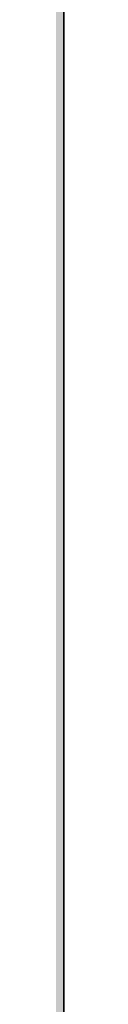
# Model space of a CAD drawing. Units: inches. Extents: x 2091 to 2899, y 967 to 2217.
# Tile 75 of 256: x 2212 to 2212, y 1105 to 1114. Entities that reach past the tile are written whole.
import ezdxf

# ---------------------------------------------------------------- set-up
doc = ezdxf.new("R2010")
doc.units = ezdxf.units.IN
doc.layers.add('A-WALL', color=7, linetype='Continuous', lineweight=35)
doc.layers.add('A-WALL-PATT', color=141, linetype='Continuous', lineweight=13, true_color=0xadddf7)

msp = doc.modelspace()

# ---------------------------------------------------------------- hatches: boundary and pattern name
at = {"layer": 'A-WALL-PATT'}
h = msp.add_hatch(color=256, dxfattribs=at)
h.dxf.hatch_style = 1
h.paths.add_polyline_path([(2212.1436, 1941.4191), (2387.6436, 1941.4191), (2387.6436, 1824.4191), (2392.1436, 1824.4191), (2392.1436, 1941.4191), (2609.6436, 1941.4191), (2609.6436, 1825.9191), (2614.1436, 1825.9191), (2614.1436, 1941.4191), (2794.1436, 1941.4191), (2794.1436, 1928.7622), (2803.1436, 1928.7622), (2803.1436, 2050.9191), (2203.1436, 2050.9191), (2203.1436, 1900.7579), (2212.1436, 1900.7579)])
h.paths.add_polyline_path([(2212.1436, 1945.9191), (2212.1436, 2041.9191), (2794.1436, 2041.9191), (2794.1436, 1945.9191), (2402.2482, 1945.9191), (2401.1024, 1945.7758), (2398.7024, 1945.7758)], flags=16)
h.paths.add_polyline_path([(2230.2299, 1948.0628), (2227.3499, 1949.5028), (2225.9099, 1951.9028), (2223.9899, 1952.8628), (2223.0299, 1955.2628), (2222.0699, 1959.5828), (2222.0699, 1963.4228), (2223.0299, 1965.6628), (2223.9899, 1965.3428), (2225.5859, 1963.8607), (2226.9115, 1964.9573), (2226.9489, 1965.9388), (2227.7783, 1966.9521), (2228.1999, 1968.8787), (2230.7099, 1964.8628), (2233.5899, 1966.3028), (2233.6073, 1966.3319), (2233.7727, 1964.9382), (2234.6338, 1963.6765), (2235.0299, 1963.9028), (2236.282, 1965.5724), (2235.9899, 1962.9428), (2237.9545, 1957.54), (2238.3899, 1957.9028), (2239.2159, 1960.3058), (2238.6546, 1966.385), (2238.6928, 1966.4381), (2238.8406, 1967.4997), (2238.7803, 1967.6875), (2238.8805, 1967.7868), (2238.6669, 1966.2518), (2239.2159, 1960.3058), (2238.3899, 1957.9028), (2236.9499, 1956.7028), (2234.5499, 1949.9828)], flags=0)
h.paths.add_polyline_path([(2278.012, 1948.0628), (2276.4964, 1947.8733), (2275.8498, 1947.6886), (2274.652, 1947.1028)], flags=0)
h.paths.add_polyline_path([(2269.852, 1955.7428), (2268.2762, 1956.6293), (2270.8673, 1956.3484), (2269.372, 1958.1428), (2268.715, 1959.1923), (2270.5698, 1958.7286), (2268.5807, 1961.9061), (2270.812, 1960.8919), (2270.812, 1963.4228), (2271.3933, 1964.7793), (2270.2918, 1966.1562), (2271.772, 1965.6628), (2272.1414, 1966.5248), (2273.9298, 1965.9286), (2275.6304, 1968.0543), (2276.3319, 1966.7219), (2276.5204, 1966.9521), (2276.942, 1968.8787), (2277.7343, 1967.6111), (2278.1399, 1969.4645), (2279.6591, 1967.0337), (2280.412, 1966.7828), (2280.9493, 1967.5888), (2281.6098, 1967.3686), (2282.1333, 1968.1538), (2282.3492, 1966.3334), (2282.3498, 1966.3326), (2283.4076, 1968.0954), (2283.7126, 1965.524), (2284.3202, 1964.6338), (2284.5118, 1964.8892), (2284.235, 1965.7048), (2284.5005, 1967.319), (2284.9079, 1965.4174), (2285.3963, 1966.0686), (2285.4328, 1966.2906), (2285.4733, 1966.1713), (2286.3539, 1967.3454), (2286.222, 1966.1582), (2287.6635, 1968.0802), (2287.714, 1968.4428), (2288.4816, 1969.0167), (2288.574, 1968.7289), (2288.9175, 1969.069), (2288.6068, 1966.8376), (2288.9287, 1963.3513), (2288.935, 1963.3568), (2288.9297, 1963.3404), (2289.0153, 1962.4139), (2290.1112, 1963.8751), (2290.1328, 1963.9426), (2290.2177, 1964.0171), (2290.1112, 1963.8751), (2289.1558, 1960.8916), (2288.594, 1959.2572), (2288.572, 1959.1028), (2289.532, 1960.5428), (2290.012, 1962.4628), (2290.1918, 1962.6427), (2289.7698, 1959.6886), (2286.8898, 1957.2886), (2284.4898, 1950.5686), (2283.3147, 1950.0463), (2283.292, 1949.9828), (2280.2901, 1948.6486), (2281.1298, 1948.6486), (2282.5698, 1948.1686), (2283.2047, 1948.0628), (2278.972, 1948.0628), (2276.092, 1949.5028), (2274.652, 1951.9028), (2272.732, 1952.8628)], flags=0)
h.paths.add_polyline_path([(2271.1589, 1958.0218), (2272.9698, 1955.8486), (2272.0098, 1960.1686), (2272.0098, 1964.0086), (2272.6244, 1965.4427), (2274.328, 1963.8607), (2275.6536, 1964.9573), (2275.6377, 1964.5391), (2277.4122, 1966.0069), (2277.033, 1965.1568), (2276.8299, 1964.9756), (2276.766, 1963.295), (2277.4496, 1962.6602), (2279.452, 1964.8628), (2282.332, 1966.3028), (2283.5298, 1966.8886), (2283.2945, 1966.7709), (2283.913, 1963.8847), (2284.8992, 1964.4483), (2284.732, 1962.9428), (2286.6966, 1957.54), (2287.132, 1957.9028), (2287.5419, 1959.0954), (2287.7794, 1958.4423), (2285.6827, 1956.6951), (2285.8765, 1959.7953), (2284.732, 1962.9428), (2284.8992, 1964.4483), (2283.913, 1963.8847), (2284.2238, 1962.4341), (2283.4244, 1963.6055), (2281.6098, 1962.5686), (2281.1298, 1960.1686), (2282.0898, 1956.3286), (2283.0498, 1952.9686), (2282.5698, 1950.5686), (2280.1698, 1948.6486), (2279.8833, 1948.7919), (2278.972, 1948.0628), (2278.972, 1949.0228), (2278.6723, 1949.3974), (2277.2898, 1950.0886), (2275.8498, 1952.4886), (2273.9298, 1953.4486), (2272.4898, 1954.8886), (2271.9216, 1954.8886), (2271.772, 1955.2628)], flags=0)
h.paths.add_polyline_path([(2311.9941, 1955.7428), (2312.0627, 1955.6742), (2312.0551, 1955.7085)], flags=0)
h.paths.add_polyline_path([(2331.9561, 1963.9518), (2333.3961, 1965.3918), (2331.0771, 1963.3568), (2330.9986, 1963.1115)], flags=0)
h.paths.add_polyline_path([(2310.5541, 1954.3028), (2307.0398, 1956.2799), (2310.7629, 1955.8763), (2312.4741, 1953.8228), (2313.4341, 1951.4228), (2315.3541, 1950.4628), (2316.7941, 1948.0628), (2317.4661, 1947.7268), (2319.3687, 1947.9646), (2317.7541, 1949.9828), (2317.5695, 1950.6105), (2316.7941, 1951.9028), (2314.8741, 1952.8628), (2313.9141, 1955.2628), (2311.5141, 1958.1428), (2309.3755, 1961.5592), (2311.5141, 1960.3371), (2311.5141, 1961.9828), (2310.6047, 1963.1196), (2311.7266, 1962.4785), (2312.4183, 1964.0926), (2312.256, 1964.2955), (2313.1941, 1963.9828), (2313.9141, 1965.6628), (2314.6468, 1965.4186), (2315.3541, 1966.3028), (2316.7941, 1967.7428), (2316.1574, 1966.9469), (2317.0341, 1965.2819), (2317.2226, 1965.5121), (2317.777, 1968.0458), (2318.4741, 1966.7219), (2318.6626, 1966.9521), (2319.0842, 1968.8787), (2321.207, 1965.4821), (2322.1614, 1966.9137), (2322.5541, 1966.7828), (2322.786, 1967.1306), (2322.8816, 1966.3243), (2323.312, 1965.7217), (2323.6513, 1965.8914), (2324.3965, 1967.1334), (2324.6569, 1964.9382), (2324.972, 1964.4766), (2325.3873, 1967.0015), (2325.9408, 1964.4183), (2327.2289, 1966.1358), (2327.1663, 1965.5724), (2328.0591, 1966.7628), (2328.2246, 1966.2475), (2329.668, 1967.6769), (2329.6646, 1967.6875), (2329.7648, 1967.7868), (2329.5511, 1966.2518), (2330.1001, 1960.3058), (2329.3328, 1958.0735), (2329.3131, 1957.9352), (2329.6341, 1958.2028), (2330.2341, 1959.1028), (2330.7141, 1961.0228), (2331.0341, 1961.3428), (2330.7141, 1959.1028), (2329.6341, 1958.2028), (2329.2741, 1957.6628), (2327.7121, 1956.3611), (2325.4341, 1949.9828), (2324.3338, 1949.4937), (2323.9941, 1948.5428), (2319.6741, 1946.6228), (2316.7941, 1948.0628), (2315.3541, 1950.4628), (2313.4341, 1951.4228)], flags=0)
h.paths.add_polyline_path([(2321.3357, 1947.952), (2321.1141, 1948.0628), (2321.1141, 1949.0228), (2319.1941, 1951.4228), (2316.7941, 1959.5828), (2316.6632, 1959.5828), (2315.3541, 1958.1428), (2314.3941, 1958.1428), (2313.1483, 1958.7091), (2312.9541, 1959.5828), (2312.9541, 1960.8919), (2315.8341, 1959.5828), (2316.6632, 1959.5828), (2317.3147, 1960.2994), (2315.0302, 1962.4207), (2316.3558, 1963.5173), (2316.3723, 1963.9516), (2316.4702, 1963.8607), (2317.7958, 1964.9573), (2317.7552, 1963.8897), (2319.1751, 1965.1568), (2319.4984, 1965.8814), (2321.1141, 1965.3428), (2323.2359, 1962.3724), (2325.6863, 1963.7726), (2325.5428, 1962.4806), (2325.1988, 1963.494), (2324.4785, 1963.0824), (2324.926, 1960.9941), (2324.0781, 1962.2365), (2322.4148, 1961.286), (2322.0741, 1959.5828), (2323.0341, 1955.7428), (2323.9941, 1952.3828), (2323.5141, 1949.9828), (2322.1427, 1948.8856), (2322.0741, 1948.5428)], flags=0)
h.paths.add_polyline_path([(2320.2075, 1963.3375), (2320.1541, 1963.4228), (2320.3941, 1963.5428)], flags=0)
h.paths.add_polyline_path([(2353.8505, 1965.8105), (2354.0305, 1965.7505), (2354.3305, 1966.4505), (2354.3305, 1966.9305)], flags=0)
h.paths.add_polyline_path([(2359.0206, 1969.0264), (2359.0984, 1968.9019), (2359.2335, 1969.5195), (2359.2335, 1969.9995)], flags=0)
h.paths.add_polyline_path([(2358.2567, 1966.6817), (2357.9836, 1966.348), (2358.2113, 1966.1462), (2358.4105, 1966.3896)], flags=0)
h.paths.add_polyline_path([(2357.7685, 1966.0588), (2357.7322, 1965.105), (2357.751, 1965.1206), (2357.7695, 1965.6065), (2357.7695, 1966.0578)], flags=0)
h.paths.add_polyline_path([(2359.1115, 1965.3045), (2359.1115, 1964.8245), (2359.8445, 1966.4675), (2359.8445, 1966.9475)], flags=0)
h.paths.add_polyline_path([(2360.2237, 1966.6214), (2360.6985, 1969.3625), (2360.6985, 1969.8425), (2360.2105, 1967.0255), (2360.2105, 1966.6425)], flags=0)
h.paths.add_polyline_path([(2363.4505, 1967.8905), (2363.4505, 1968.3705), (2362.4905, 1966.9305), (2362.656, 1966.6988)], flags=0)
h.paths.add_polyline_path([(2364.4755, 1966.0788), (2365.8505, 1968.3705), (2365.8505, 1968.8505), (2364.428, 1966.4796)], flags=0)
h.paths.add_polyline_path([(2366.3135, 1965.8525), (2366.3667, 1965.6958), (2366.8025, 1968.3455), (2366.8025, 1968.8255)], flags=0)
h.paths.add_polyline_path([(2367.1653, 1965.8035), (2367.2905, 1966.9305), (2367.2905, 1967.4105), (2367.1027, 1965.7201)], flags=0)
h.paths.add_polyline_path([(2370.0365, 1959.9735), (2371.0135, 1963.0245), (2371.0135, 1963.5045), (2370.0365, 1960.4535)], flags=0)
h.paths.add_polyline_path([(2371.6105, 1960.2105), (2372.5705, 1961.6505), (2372.5705, 1962.1305), (2371.8025, 1960.9785)], flags=0)
h.paths.add_polyline_path([(2350.8737, 1956.0051), (2351.9305, 1955.8905), (2354.4905, 1953.3305), (2353.8505, 1954.9305), (2351.4505, 1957.8105), (2347.9355, 1963.4255), (2347.9355, 1963.9055), (2351.4505, 1958.2905), (2353.7051, 1955.585), (2352.8905, 1959.2505), (2352.8905, 1959.7305), (2352.8905, 1961.9248), (2356.7305, 1959.7305), (2358.4545, 1961.6268), (2354.8105, 1965.0105), (2355.0309, 1965.2859), (2358.6911, 1961.8871), (2361.5305, 1965.0105), (2364.3765, 1966.4335), (2364.5244, 1965.1869), (2365.4545, 1963.8242), (2365.8811, 1964.068), (2365.3705, 1966.4505), (2365.3705, 1966.9305), (2366.8105, 1960.2105), (2366.8105, 1959.7305), (2366.3887, 1952.9814), (2367.7705, 1956.8505), (2368.6412, 1957.5761), (2366.8105, 1962.6105), (2366.8105, 1963.0905), (2368.7752, 1957.6877), (2369.2105, 1958.0505), (2370.0016, 1960.3519), (2369.4752, 1966.0527), (2369.5135, 1966.1058), (2369.5142, 1966.1109), (2369.4752, 1966.5327), (2369.5135, 1966.5858), (2369.6146, 1967.3126), (2369.1825, 1968.6585), (2369.1825, 1969.1385), (2369.601, 1967.8352), (2369.7012, 1967.9345), (2369.7179, 1968.0547), (2370.1452, 1968.3741), (2369.7787, 1968.0112), (2369.7012, 1967.4545), (2370.4682, 1968.214), (2369.6749, 1967.2658), (2369.5142, 1966.1109), (2370.0365, 1960.4535), (2370.0365, 1959.9735), (2369.4418, 1958.2432), (2370.6505, 1959.2505), (2371.0458, 1962.0176), (2371.1305, 1962.1305), (2370.6505, 1958.7705), (2367.7705, 1956.3705), (2365.3705, 1949.6505), (2362.0791, 1948.1876), (2363.4505, 1947.7305), (2361.0505, 1947.7305), (2360.0905, 1947.7305), (2357.1039, 1947.3572), (2360.0905, 1948.2105), (2358.1705, 1949.1705), (2356.7305, 1951.5705), (2354.8105, 1952.5305), (2351.9305, 1955.4105)], flags=0)
h.paths.add_polyline_path([(2361.0505, 1948.6905), (2359.1305, 1951.0905), (2356.7305, 1959.2505), (2355.7705, 1959.2505), (2352.8905, 1960.5596), (2352.8905, 1961.4448), (2355.8905, 1959.7305), (2356.7305, 1959.7305), (2356.8372, 1959.3678), (2361.5305, 1964.5305), (2363.2484, 1965.3894), (2364.9253, 1963.0418), (2362.4905, 1961.6505), (2362.0639, 1959.5172), (2362.9705, 1955.8905), (2363.9305, 1952.5305), (2363.9305, 1952.0505), (2363.4505, 1949.6505), (2361.0505, 1947.7305)], flags=0)
h.paths.add_polyline_path([(2359.1305, 1951.5705), (2359.2905, 1951.3705), (2361.0505, 1954.4505), (2361.0505, 1954.9305)], flags=0)
h.paths.add_polyline_path([(2357.2195, 1966.5455), (2356.7925, 1968.8145), (2356.7925, 1969.2945), (2357.2195, 1967.0255)], flags=0)
h.paths.add_polyline_path([(2361.0505, 1954.4505), (2361.5305, 1958.7705), (2361.5305, 1959.2505), (2361.0505, 1954.9305)], flags=0)
h.paths.add_polyline_path([(2402.5483, 1948.4861), (2402.3024, 1948.4158), (2402.5904, 1948.4158)], flags=0)
h.paths.add_polyline_path([(2394.1424, 1956.0958), (2395.6851, 1954.5532), (2396.7205, 1953.9707), (2396.0624, 1955.6158), (2395.2414, 1956.6011), (2395.8789, 1956.4417), (2395.1024, 1959.9358), (2395.1024, 1963.7758), (2396.0624, 1966.0158), (2397.0224, 1965.6958), (2398.6185, 1964.2138), (2399.9441, 1965.3103), (2399.9814, 1966.2918), (2400.8109, 1967.3052), (2401.2325, 1969.2317), (2403.5379, 1965.543), (2403.942, 1967.3893), (2404.7024, 1967.1358), (2405.4603, 1966.0748), (2406.6224, 1966.6558), (2406.6399, 1966.6849), (2406.8052, 1965.2912), (2406.9257, 1965.1147), (2407.3424, 1964.9758), (2407.8743, 1965.7737), (2408.1691, 1964.3981), (2409.3146, 1965.9254), (2409.2175, 1965.0511), (2409.4452, 1963.1312), (2410.3064, 1961.8695), (2410.7024, 1962.0958), (2411.4423, 1963.0823), (2411.1654, 1963.8978), (2411.6164, 1966.6398), (2411.7254, 1966.7911), (2411.8732, 1967.8527), (2411.8129, 1968.0405), (2411.9131, 1968.1398), (2411.6994, 1966.6048), (2412.2484, 1960.6588), (2413.2254, 1963.7098), (2414.3779, 1964.7212), (2414.5132, 1965.6927), (2414.4529, 1965.8805), (2414.5531, 1965.9798), (2414.3779, 1964.7212), (2414.5198, 1964.8457), (2414.3654, 1964.6311), (2414.3394, 1964.4448), (2414.8884, 1958.4988), (2414.0624, 1956.0958), (2412.6224, 1954.8958), (2410.1714, 1948.0329), (2410.0167, 1948.0844), (2405.9024, 1946.2558), (2405.9024, 1947.2158), (2405.2043, 1948.0886), (2404.2224, 1948.4158), (2403.2624, 1948.4158), (2400.3824, 1949.8558), (2399.6624, 1951.0558), (2397.9824, 1952.7358), (2397.0224, 1953.2158), (2395.6851, 1954.5532), (2392.6568, 1956.2569)], flags=0)
h.paths.add_polyline_path([(2409.0857, 1964.4074), (2409.1304, 1964.2757), (2409.2624, 1964.4958)], flags=0)
h.paths.add_polyline_path([(2397.7424, 1961.6158), (2398.7024, 1963.8558), (2399.6624, 1963.5358), (2401.4266, 1965.741), (2401.7914, 1966.5588), (2402.0714, 1965.0708), (2402.8355, 1964.3934), (2403.2624, 1964.9149), (2403.3381, 1964.7711), (2402.6155, 1963.9762), (2402.4986, 1960.9022), (2403.543, 1959.9325), (2404.4132, 1960.8897), (2404.7024, 1962.3358), (2407.9163, 1964.1724), (2409.5202, 1961.9269), (2410.9871, 1957.893), (2411.4224, 1958.2558), (2412.048, 1960.0756), (2412.4103, 1959.0791), (2411.6756, 1958.4668), (2411.6624, 1958.2558), (2411.6261, 1958.4255), (2409.9824, 1957.0558), (2407.5824, 1950.3358), (2403.2624, 1948.4158), (2403.2624, 1949.3758), (2401.3424, 1951.7758), (2399.4165, 1958.324), (2397.7424, 1959.0849), (2397.7424, 1959.9701), (2397.1024, 1960.3358), (2397.7424, 1960.0449)], flags=0)
h.paths.add_polyline_path([(2405.9024, 1952.9758), (2405.9504, 1953.4078), (2406.0167, 1953.1758)], flags=0)
h.paths.add_polyline_path([(2449.8178, 1967.114), (2449.7523, 1967.1358), (2449.7937, 1967.0779)], flags=0)
h.paths.add_polyline_path([(2451.6977, 1966.6181), (2451.7409, 1966.6901), (2451.6921, 1966.6657)], flags=0)
h.paths.add_polyline_path([(2454.3436, 1965.7376), (2455.7523, 1967.6158), (2455.9923, 1968.0958), (2454.3645, 1965.9254)], flags=0)
h.paths.add_polyline_path([(2457.5473, 1968.8638), (2457.7873, 1969.3438), (2457.0543, 1968.7958), (2457.0076, 1968.4603)], flags=0)
h.paths.add_polyline_path([(2456.9218, 1967.8567), (2456.8022, 1968.229), (2456.723, 1967.6598)], flags=0)
h.paths.add_polyline_path([(2457.3023, 1967.3768), (2457.5423, 1967.8568), (2456.8103, 1966.8398), (2456.7405, 1966.7002), (2456.749, 1966.6081)], flags=0)
h.paths.add_polyline_path([(2458.2753, 1963.7098), (2458.1553, 1963.3352), (2460.3543, 1965.2648), (2460.5943, 1965.7448)], flags=0)
h.paths.add_polyline_path([(2458.3923, 1962.8158), (2458.3641, 1962.6182), (2459.5923, 1964.2558), (2459.8323, 1964.7358)], flags=0)
h.paths.add_polyline_path([(2459.3523, 1962.8158), (2459.2723, 1962.4958), (2460.0723, 1963.2958), (2460.3123, 1963.7758)], flags=0)
h.paths.add_polyline_path([(2458.6803, 1960.6078), (2458.6323, 1960.4158), (2459.5923, 1961.8558), (2459.8323, 1962.3358)], flags=0)
h.paths.add_polyline_path([(2437.8382, 1956.2427), (2439.1923, 1956.0958), (2441.3523, 1953.9358), (2440.8723, 1955.1358), (2438.4723, 1958.0158), (2438.0716, 1958.656), (2438.7123, 1958.4958), (2440.6396, 1956.1831), (2439.9123, 1959.4558), (2439.9123, 1963.2958), (2441.3523, 1966.6558), (2441.5923, 1967.1358), (2441.1123, 1966.0158), (2442.0723, 1965.6958), (2443.989, 1968.0917), (2444.2413, 1966.7508), (2444.9168, 1966.1519), (2445.6766, 1967.0801), (2446.2553, 1969.7248), (2446.4953, 1970.2048), (2446.2824, 1969.2317), (2447.3627, 1967.5033), (2447.7203, 1969.5678), (2447.9603, 1970.0478), (2447.4855, 1967.3068), (2448.7923, 1965.2158), (2448.4723, 1964.8638), (2448.5523, 1964.7358), (2451.4521, 1966.1857), (2451.6151, 1964.8112), (2452.3079, 1963.7962), (2453.2345, 1964.3257), (2454.0723, 1960.4158), (2453.6287, 1953.3177), (2454.7923, 1956.5758), (2455.0323, 1957.0558), (2455.7188, 1957.6279), (2453.8323, 1962.8158), (2453.941, 1963.7936), (2453.3353, 1965.5778), (2453.8243, 1968.5508), (2454.0643, 1969.0308), (2453.5753, 1966.0578), (2454.0403, 1964.6879), (2453.8323, 1962.8158), (2455.7188, 1957.6279), (2456.3672, 1958.1682), (2457.0583, 1960.1788), (2457.2983, 1960.6588), (2456.4723, 1958.2558), (2457.7177, 1959.2937), (2457.6723, 1958.9758), (2454.89, 1956.6572), (2453.6141, 1953.0849), (2453.5923, 1952.7358), (2453.3523, 1952.2558), (2453.3596, 1952.3722), (2452.6323, 1950.3358), (2452.3923, 1949.8558), (2449.2038, 1948.4387), (2450.7123, 1947.9358), (2448.0723, 1947.9358), (2447.1123, 1947.9358), (2444.5523, 1947.6158), (2447.1996, 1948.3722), (2445.1923, 1949.3758), (2443.7523, 1951.7758), (2441.8323, 1952.7358), (2438.9523, 1955.6158)], flags=0)
h.paths.add_polyline_path([(2443.9923, 1959.9358), (2444.0403, 1959.7726), (2444.1216, 1959.862)], flags=0)
h.paths.add_polyline_path([(2442.9123, 1959.9358), (2443.0323, 1959.9358), (2442.4457, 1960.2025)], flags=0)
h.paths.add_polyline_path([(2444.9829, 1965.0197), (2445.2793, 1965.2648), (2445.5193, 1965.7448), (2444.994, 1965.3103)], flags=0)
h.paths.add_polyline_path([(2446.1333, 1965.0298), (2446.3304, 1965.4715), (2444.9703, 1964.2578), (2444.7303, 1963.7778)], flags=0)
h.paths.add_polyline_path([(2442.7923, 1959.4558), (2443.7523, 1959.4558), (2446.1523, 1951.2958), (2446.4123, 1951.7508), (2446.3923, 1951.7758), (2448.0806, 1954.7303), (2448.5523, 1958.9758), (2441.8323, 1965.2158), (2442.1549, 1965.6191), (2448.7923, 1959.4558), (2448.3123, 1955.1358), (2448.0723, 1954.6558), (2446.4123, 1951.7508), (2448.3123, 1949.3758), (2448.3123, 1948.4158), (2450.5409, 1950.1987), (2450.9523, 1952.2558), (2449.9923, 1955.6158), (2449.0323, 1959.4558), (2449.5123, 1961.8558), (2449.7523, 1962.3358), (2449.6749, 1961.9487), (2452.9945, 1963.8457), (2453.0644, 1963.5194), (2452.8846, 1963.7829), (2449.6749, 1961.9487), (2449.2723, 1959.9358), (2450.2323, 1956.0958), (2451.1923, 1952.7358), (2450.7123, 1950.3358), (2450.4723, 1949.8558), (2448.0723, 1947.9358), (2448.0723, 1948.5358), (2445.4323, 1949.8558), (2443.9923, 1952.2558), (2442.0723, 1953.2158), (2441.1123, 1955.6158), (2440.1523, 1959.9358), (2440.1523, 1960.6558)], flags=0)
h.paths.add_polyline_path([(2456.6923, 1966.9858), (2457.6083, 1968.0808), (2457.8483, 1968.5608), (2456.9323, 1967.4658)], flags=0)
h.paths.add_polyline_path([(2489.8966, 1966.5802), (2489.9429, 1966.1893), (2490.7475, 1967.5302), (2491.3191, 1968.9512)], flags=0)
h.paths.add_polyline_path([(2473.5625, 1956.4071), (2477.14, 1956.0193), (2476.9553, 1956.2408), (2475.108, 1957.2801), (2476.3475, 1956.9702), (2475.1869, 1958.8242), (2476.9191, 1958.3912), (2475.4116, 1960.7993), (2477.7875, 1959.7193), (2477.7875, 1962.2502), (2477.6374, 1962.4379), (2477.8226, 1962.3321), (2478.3591, 1963.5841), (2478.3591, 1963.6712), (2477.3243, 1964.9646), (2478.7148, 1964.5011), (2479.3191, 1965.9112), (2480.2791, 1965.5912), (2481.784, 1967.4722), (2482.1165, 1965.7052), (2482.8806, 1965.0278), (2483.2093, 1965.4294), (2483.2202, 1965.7151), (2483.0759, 1965.989), (2483.7118, 1966.7658), (2484.1305, 1968.6792), (2484.7021, 1970.1002), (2484.4892, 1969.1271), (2486.5029, 1965.9051), (2487.3875, 1965.6102), (2488.1534, 1966.7591), (2488.717, 1965.9701), (2489.2001, 1966.2116), (2489.3307, 1965.111), (2490.3939, 1963.6225), (2490.6608, 1963.775), (2490.4939, 1964.5536), (2490.9231, 1963.9248), (2491.3191, 1964.1512), (2491.3334, 1964.1702), (2491.2105, 1964.5322), (2491.2818, 1964.9655), (2491.4258, 1964.2934), (2494.0765, 1967.8276), (2494.4979, 1966.5149), (2494.5982, 1966.6142), (2494.6895, 1967.2702), (2495.1067, 1967.5822), (2495.1298, 1967.7481), (2495.0696, 1967.9359), (2495.1698, 1968.0351), (2495.0318, 1967.0436), (2495.7538, 1967.7587), (2494.9821, 1966.6864), (2494.9561, 1966.5002), (2495.479, 1960.8369), (2495.9105, 1962.1842), (2496.4821, 1963.6052), (2496.0727, 1962.3266), (2496.7689, 1962.9375), (2496.5991, 1962.7112), (2496.1191, 1959.3512), (2496.7329, 1960.2718), (2496.9875, 1961.2902), (2497.5591, 1962.7112), (2497.0791, 1960.7912), (2496.5075, 1959.3702), (2495.5475, 1957.9302), (2492.7588, 1955.6064), (2490.8391, 1950.2312), (2490.2675, 1948.8102), (2485.9475, 1946.8902), (2483.0675, 1948.3302), (2481.6275, 1950.7302), (2479.7075, 1951.6902), (2476.8275, 1954.5702)], flags=0)
h.paths.add_polyline_path([(2485.577, 1948.3134), (2485.5591, 1948.3112), (2485.5788, 1948.3112)], flags=0)
h.paths.add_polyline_path([(2478.6451, 1954.5512), (2478.109, 1956.9633), (2479.3191, 1955.5112), (2480.2791, 1953.1112), (2482.1991, 1952.1512), (2483.6391, 1949.7512), (2486.5191, 1948.3112), (2486.5191, 1949.2712), (2484.7393, 1951.4959), (2484.0275, 1950.2502), (2481.6275, 1958.4102), (2482.3751, 1959.2327), (2482.1991, 1959.8312), (2483.1976, 1960.9295), (2479.7075, 1964.1702), (2480.6034, 1965.2901), (2481.8752, 1964.1091), (2482.6664, 1964.7636), (2482.6154, 1963.4218), (2482.9892, 1963.0747), (2484.0085, 1963.9842), (2484.6836, 1965.4975), (2484.5801, 1965.4052), (2485.3573, 1967.1471), (2485.1206, 1965.7812), (2486.4275, 1963.6902), (2488.1454, 1964.5492), (2489.8223, 1962.2016), (2490.7475, 1962.7302), (2491.9997, 1964.3998), (2492.076, 1965.0873), (2492.2129, 1964.6841), (2492.4854, 1965.0474), (2492.2791, 1963.1912), (2494.2438, 1957.7884), (2494.5625, 1958.054), (2494.9335, 1959.1332), (2495.5051, 1960.5542), (2494.6791, 1958.1512), (2494.1075, 1956.7302), (2494.5625, 1958.054), (2493.4085, 1957.0923), (2491.7075, 1961.7702), (2491.9997, 1964.3998), (2490.7475, 1962.7302), (2487.712, 1960.9957), (2487.4791, 1959.8312), (2488.4391, 1955.9912), (2489.3991, 1952.6312), (2488.9191, 1950.2312), (2488.5769, 1949.9574), (2488.3475, 1948.8102), (2487.6517, 1948.2536), (2487.4791, 1948.3112), (2486.5191, 1948.3112), (2483.6391, 1949.7512), (2482.1991, 1952.1512), (2480.2791, 1953.1112), (2478.8391, 1954.5512)], flags=0)
h.paths.add_polyline_path([(2526.6483, 1966.9875), (2526.5173, 1967.0312), (2526.6001, 1966.9153)], flags=0)
h.paths.add_polyline_path([(2528.4706, 1966.4467), (2528.5745, 1966.6197), (2528.4571, 1966.561)], flags=0)
h.paths.add_polyline_path([(2534.1333, 1967.4962), (2534.1567, 1967.5428), (2534.0598, 1967.4083)], flags=0)
h.paths.add_polyline_path([(2536.1619, 1964.0506), (2535.1573, 1962.7112), (2535.1009, 1962.3159), (2536.1173, 1963.6712), (2536.4205, 1964.2775)], flags=0)
h.paths.add_polyline_path([(2535.1573, 1959.8312), (2536.1173, 1961.2712), (2536.5973, 1962.2312), (2535.2533, 1960.2152)], flags=0)
h.paths.add_polyline_path([(2513.249, 1956.2848), (2516.2212, 1955.9626), (2514.9973, 1957.4312), (2514.1958, 1958.7115), (2515.4773, 1958.3912), (2516.9319, 1956.6457), (2516.4373, 1958.8712), (2516.4373, 1962.7112), (2516.8727, 1963.727), (2515.3464, 1965.6348), (2517.3973, 1964.9512), (2517.8773, 1966.0712), (2518.3573, 1967.0312), (2517.8773, 1965.9112), (2518.8373, 1965.5912), (2520.4866, 1967.6527), (2520.7663, 1966.1662), (2521.5304, 1965.4887), (2521.7814, 1965.7954), (2521.8009, 1966.3073), (2521.4778, 1966.9209), (2521.2463, 1967.1262), (2521.1777, 1967.4909), (2521.4778, 1966.9209), (2522.0104, 1966.4487), (2522.2574, 1966.7504), (2522.7803, 1969.1402), (2523.2603, 1970.1002), (2523.0474, 1969.1271), (2524.6731, 1966.5259), (2526.0373, 1966.0712), (2526.7952, 1965.0101), (2527.9771, 1965.601), (2528.1401, 1964.2266), (2528.6646, 1963.4582), (2529.3886, 1963.8719), (2529.3297, 1964.147), (2529.4813, 1963.9248), (2529.8773, 1964.1512), (2529.984, 1964.2934), (2529.7891, 1965.2032), (2530.0624, 1964.3979), (2532.8025, 1968.0513), (2533.1478, 1966.9759), (2533.248, 1967.0751), (2533.3393, 1967.7312), (2533.6728, 1967.9805), (2533.728, 1968.0351), (2533.5143, 1966.5002), (2534.0247, 1960.9725), (2534.5603, 1962.6452), (2535.0403, 1963.6052), (2534.0633, 1960.5542), (2533.2373, 1958.1512), (2534.2882, 1959.0268), (2534.1973, 1958.3912), (2531.5126, 1956.1539), (2529.3973, 1950.2312), (2528.9173, 1949.2712), (2526.4488, 1948.174), (2527.4773, 1947.8312), (2530.3573, 1947.3512), (2524.5973, 1947.3512), (2521.7173, 1948.7912), (2520.2773, 1951.1912), (2518.3573, 1952.1512), (2515.4773, 1955.0312)], flags=0)
h.paths.add_polyline_path([(2523.9348, 1967.1903), (2523.6195, 1966.4837), (2523.7705, 1966.2421)], flags=0)
h.paths.add_polyline_path([(2518.8373, 1953.1112), (2517.8773, 1955.5112), (2516.885, 1959.9768), (2516.9173, 1959.9621), (2516.9173, 1962.0254), (2520.7573, 1959.8312), (2522.0249, 1961.2255), (2518.3573, 1964.6312), (2519.0026, 1965.4377), (2520.4334, 1964.1091), (2521.3011, 1964.8269), (2521.2452, 1963.3553), (2525.6383, 1959.276), (2526.0373, 1961.2712), (2529.3973, 1963.1912), (2530.6495, 1964.8607), (2530.6647, 1964.9976), (2530.692, 1964.9173), (2531.0878, 1965.4451), (2530.946, 1964.1689), (2530.692, 1964.9173), (2529.3973, 1963.1912), (2526.3625, 1961.457), (2526.0373, 1959.8312), (2526.9973, 1955.9912), (2527.9573, 1952.6312), (2527.4773, 1950.2312), (2527.1345, 1949.9569), (2526.9739, 1949.1541), (2526.6973, 1949.0312), (2524.5973, 1947.3512), (2524.5973, 1948.3112), (2524.2773, 1948.7112), (2522.1973, 1949.7512), (2520.7573, 1952.1512)], flags=0)
h.paths.add_polyline_path([(2520.2773, 1958.8712), (2520.8533, 1959.5048), (2523.1573, 1951.6712), (2524.6139, 1954.2201), (2524.5973, 1954.0712), (2522.6773, 1950.7112)], flags=0)
h.paths.add_polyline_path([(2559.3709, 1966.3112), (2559.3984, 1966.3249), (2559.4019, 1966.3453)], flags=0)
h.paths.add_polyline_path([(2549.7709, 1957.1912), (2552.6509, 1954.3112), (2552.134, 1955.6035), (2550.6109, 1957.4312), (2547.0959, 1963.0462), (2545.7759, 1965.2062), (2549.2909, 1959.5912), (2551.6909, 1956.7112), (2550.7929, 1960.7521), (2550.7309, 1960.7803), (2550.7309, 1964.8712), (2551.6909, 1967.1112), (2552.6509, 1966.7912), (2554.247, 1965.3091), (2555.0343, 1965.9603), (2555.5817, 1966.6446), (2555.6099, 1967.3872), (2556.4394, 1968.4005), (2556.861, 1970.3271), (2559.3709, 1966.3112), (2560.6909, 1964.1512), (2562.4088, 1965.0101), (2561.6509, 1966.0712), (2560.3309, 1968.2312), (2561.7585, 1966.2325), (2562.3472, 1967.1156), (2562.4337, 1966.3866), (2563.1278, 1965.3696), (2563.5709, 1965.5912), (2563.5884, 1965.6202), (2563.3625, 1967.5235), (2563.7225, 1965.8438), (2565.06, 1968.073), (2564.7329, 1965.1287), (2565.1176, 1963.3334), (2567.4446, 1966.4361), (2567.3156, 1967.8333), (2567.3538, 1967.8864), (2567.5016, 1968.9481), (2567.4413, 1969.1359), (2567.5416, 1969.2351), (2567.3279, 1967.7002), (2567.8769, 1961.7542), (2568.7467, 1964.4703), (2568.6356, 1965.6733), (2568.6738, 1965.7264), (2568.8216, 1966.7881), (2568.7613, 1966.9759), (2568.8616, 1967.0751), (2568.6479, 1965.5402), (2568.7261, 1964.693), (2568.8539, 1964.8052), (2568.7467, 1964.4703), (2568.8172, 1963.7063), (2568.9709, 1963.9112), (2568.8661, 1963.1773), (2569.1969, 1959.5942), (2568.3709, 1957.1912), (2566.9309, 1955.9912), (2564.6203, 1949.5214), (2564.6509, 1949.5112), (2564.6166, 1949.5112), (2564.5309, 1949.2712), (2560.2109, 1947.3512), (2557.3309, 1948.7912), (2556.0452, 1950.934), (2556.0109, 1950.9512), (2555.8566, 1951.2083), (2553.9709, 1952.1512), (2551.0909, 1955.0312), (2546.6501, 1957.5295)], flags=0)
h.paths.add_polyline_path([(2567.0258, 1959.3302), (2567.035, 1959.3049), (2567.0509, 1959.3512)], flags=0)
h.paths.add_polyline_path([(2551.9683, 1962.5184), (2553.0109, 1964.9512), (2553.9709, 1964.6312), (2555.567, 1963.1491), (2556.8926, 1964.2456), (2556.9299, 1965.2272), (2557.144, 1965.4887), (2556.4201, 1966.1306), (2556.3914, 1966.105), (2556.3799, 1966.1662), (2556.4201, 1966.1306), (2556.9519, 1966.6052), (2557.0921, 1966.9195), (2557.5709, 1966.0102), (2557.7594, 1966.2405), (2557.4179, 1964.6802), (2556.8926, 1964.2456), (2556.8071, 1961.9976), (2560.6909, 1958.3912), (2560.6355, 1957.8927), (2560.8109, 1957.1912), (2561.7709, 1953.8312), (2561.2909, 1951.4312), (2559.1104, 1949.6868), (2559.1565, 1949.6292), (2563.0265, 1951.3492), (2562.6109, 1949.2712), (2560.2109, 1947.3512), (2560.2109, 1948.3112), (2559.2509, 1949.5112), (2558.8909, 1949.5112), (2558.8909, 1949.9612), (2558.2909, 1950.7112), (2558.0537, 1951.5177), (2556.9709, 1952.8712), (2555.0679, 1959.3415), (2552.0509, 1961.0654), (2552.0509, 1962.4712)], flags=0)
h.paths.add_polyline_path([(2588.33, 1958.3912), (2588.6102, 1958.111), (2588.5534, 1958.3669)], flags=0)
h.paths.add_polyline_path([(2594.7455, 1950.4931), (2593.9575, 1953.172), (2593.13, 1954.5512), (2591.21, 1955.5112), (2590.25, 1957.9112), (2588.309, 1960.2404), (2586.1773, 1961.2093), (2587.85, 1960.7912), (2587.2534, 1961.7442), (2588.4413, 1961.0654), (2588.4413, 1962.6555), (2588.4217, 1962.6653), (2588.4413, 1962.7112), (2586.914, 1964.6203), (2588.8771, 1963.728), (2589.29, 1964.6915), (2589.29, 1966.0712), (2590.25, 1968.3112), (2591.21, 1967.9912), (2592.8061, 1966.5091), (2594.1317, 1967.6056), (2594.169, 1968.5872), (2594.9985, 1969.6005), (2595.4201, 1971.5271), (2597.93, 1967.5112), (2600.81, 1968.9512), (2600.8275, 1968.9802), (2600.9928, 1967.5866), (2601.854, 1966.3248), (2602.1071, 1966.4695), (2602.2364, 1967.2551), (2602.3567, 1966.6934), (2603.5022, 1968.2207), (2603.21, 1965.5912), (2605.1747, 1960.1884), (2605.5069, 1960.4652), (2605.026, 1965.6733), (2605.0642, 1965.7264), (2605.212, 1966.7881), (2605.1517, 1966.9759), (2605.252, 1967.0751), (2605.3433, 1967.7312), (2605.9529, 1968.1869), (2605.8748, 1969.0333), (2605.913, 1969.0864), (2606.0608, 1970.1481), (2606.0005, 1970.3359), (2606.1007, 1970.4351), (2605.887, 1968.9002), (2606.436, 1962.9542), (2605.61, 1960.5512), (2605.997, 1960.8737), (2606.5643, 1962.6452), (2608.2415, 1964.1169), (2608.01, 1963.1912), (2607.05, 1961.7512), (2606.6315, 1961.4024), (2606.2013, 1958.3912), (2603.3213, 1955.9912), (2600.9213, 1949.2712), (2596.6013, 1947.3512), (2593.7213, 1948.7912), (2592.8573, 1950.2312), (2592.65, 1950.2312)], flags=0)
h.paths.add_polyline_path([(2596.6013, 1947.3512), (2596.6013, 1948.3112), (2594.6813, 1950.7112), (2596.155, 1953.29), (2595.53, 1954.0712), (2593.1992, 1961.996), (2592.6513, 1962.5047), (2591.7802, 1963.0025), (2593.283, 1964.2456), (2593.3203, 1965.2272), (2594.1498, 1966.2405), (2594.5714, 1968.1671), (2596.1827, 1965.589), (2596.9513, 1966.4345), (2598.0413, 1966.0712), (2598.7992, 1965.0101), (2599.9613, 1965.5912), (2599.9788, 1965.6202), (2600.1441, 1964.2266), (2601.0053, 1962.9648), (2601.4013, 1963.1912), (2602.6535, 1964.8607), (2602.3613, 1962.2312), (2603.7927, 1958.2947), (2601.9776, 1953.2124), (2601.9462, 1952.7095), (2599.4688, 1951.6084), (2599.0013, 1949.2712)], flags=0)
h.paths.add_polyline_path([(2597.5613, 1958.8712), (2597.671, 1959.4194), (2597.5951, 1958.7362)], flags=0)
h.paths.add_polyline_path([(2623.6663, 1961.2544), (2625.5192, 1960.7912), (2624.9655, 1961.6755), (2627.1992, 1960.6603), (2627.1992, 1961.1512), (2626.9592, 1962.2312), (2626.9592, 1963.4912), (2625.5823, 1965.2122), (2626.9592, 1964.4254), (2626.9592, 1965.8312), (2626.8692, 1965.8612), (2627.9192, 1968.3112), (2628.8792, 1967.9912), (2630.4752, 1966.5091), (2631.8008, 1967.6056), (2631.8382, 1968.5872), (2632.6676, 1969.6005), (2633.0892, 1971.5271), (2635.5992, 1967.5112), (2638.4792, 1968.9512), (2638.4966, 1968.9802), (2638.662, 1967.5866), (2639.1763, 1966.833), (2639.7802, 1967.8396), (2640.0258, 1966.6934), (2641.1713, 1968.2207), (2640.8792, 1965.5912), (2641.1143, 1964.9446), (2641.4113, 1965.3407), (2641.3081, 1964.4116), (2642.8438, 1960.1884), (2643.2792, 1960.5512), (2644.0847, 1962.8947), (2643.7839, 1966.1533), (2643.8068, 1966.1852), (2643.6007, 1968.4181), (2643.5228, 1968.6606), (2643.7299, 1970.1481), (2643.6696, 1970.3359), (2643.7698, 1970.4351), (2643.5562, 1968.9002), (2643.6007, 1968.4181), (2643.9096, 1967.4559), (2644.0098, 1967.5551), (2643.8117, 1966.1321), (2644.1052, 1962.9542), (2644.2388, 1961.3508), (2644.7192, 1961.7512), (2645.0329, 1962.2217), (2645.3222, 1963.1252), (2646.0764, 1963.787), (2645.0329, 1962.2217), (2644.3452, 1960.0742), (2643.5192, 1957.6712), (2642.0792, 1956.4712), (2639.7196, 1949.8644), (2639.8755, 1949.8384), (2635.3592, 1947.8312), (2632.4792, 1949.2712), (2631.0392, 1951.6712), (2629.1192, 1952.6312), (2628.1592, 1955.0312), (2625.7592, 1957.9112)], flags=0)
h.paths.add_polyline_path([(2627.8163, 1956.574), (2627.3737, 1958.5657), (2626.3763, 1959.7626), (2627.1992, 1959.3512), (2627.3737, 1958.5657), (2627.9192, 1957.9112), (2628.8792, 1955.5112), (2630.7992, 1954.5512), (2632.2392, 1952.1512), (2633.315, 1951.6132), (2631.0392, 1959.3512), (2631.4978, 1959.8557), (2630.7992, 1962.2312), (2631.4499, 1962.9469), (2630.7152, 1963.6291), (2632.0408, 1964.7256), (2632.0782, 1965.7072), (2632.2922, 1965.9687), (2631.7053, 1966.4891), (2633.1364, 1967.7661), (2633.3292, 1968.6471), (2634.6747, 1966.4943), (2635.2085, 1967.0814), (2636.7992, 1966.5512), (2637.6764, 1967.867), (2638.9939, 1966.0225), (2639.7053, 1966.429), (2641.1192, 1959.8312), (2640.9301, 1956.8057), (2639.4392, 1952.6312), (2638.2275, 1952.0926), (2637.7592, 1949.7512), (2635.3592, 1947.8312), (2635.3592, 1948.7912), (2633.4392, 1951.1912), (2633.315, 1951.6132), (2632.2392, 1952.1512), (2630.7992, 1954.5512), (2628.8792, 1955.5112)], flags=0)
h.paths.add_polyline_path([(2637.7592, 1953.8312), (2637.2792, 1955.5112), (2636.3192, 1959.3512), (2636.7992, 1961.7512), (2639.2339, 1963.1425), (2637.5571, 1965.4901), (2638.7389, 1966.081), (2638.902, 1964.7066), (2639.7631, 1963.4448), (2636.7992, 1961.7512), (2636.5325, 1960.4178), (2637.0392, 1958.3912), (2637.9992, 1955.0312)], flags=0)
h.paths.add_polyline_path([(2668.5674, 1951.4312), (2667.6074, 1953.8312), (2665.2074, 1956.7112), (2662.2939, 1961.3653), (2665.4474, 1959.5912), (2666.6474, 1958.3912), (2666.6474, 1959.9752), (2666.0583, 1960.6821), (2666.6474, 1960.3454), (2666.6474, 1961.9912), (2666.7001, 1962.1141), (2666.4074, 1963.4312), (2666.4074, 1967.2712), (2667.3674, 1969.5112), (2668.3274, 1969.1912), (2669.9235, 1967.7091), (2671.2491, 1968.8056), (2671.2864, 1969.7872), (2672.1159, 1970.8005), (2672.5375, 1972.7271), (2675.0474, 1968.7112), (2677.9274, 1970.1512), (2677.9449, 1970.1802), (2678.1102, 1968.7866), (2678.9713, 1967.5248), (2679.3674, 1967.7512), (2680.6196, 1969.4207), (2680.3274, 1966.7912), (2682.2921, 1961.3884), (2682.7274, 1961.7512), (2683.3583, 1963.5866), (2683.2321, 1964.9533), (2683.2703, 1965.0064), (2683.3932, 1965.8891), (2683.36, 1966.2492), (2683.3578, 1966.2559), (2683.3592, 1966.2572), (2682.9921, 1970.2333), (2683.0303, 1970.2864), (2683.1781, 1971.3481), (2683.1178, 1971.5359), (2683.2181, 1971.6351), (2683.0044, 1970.1002), (2683.3592, 1966.2572), (2683.4581, 1966.3551), (2683.3932, 1965.8891), (2683.4139, 1965.665), (2684.4238, 1966.8723), (2683.5534, 1964.1542), (2683.3583, 1963.5866), (2683.7934, 1958.8742), (2682.9674, 1956.4712), (2681.5274, 1955.2712), (2680.1092, 1951.3003), (2680.0849, 1950.9116), (2679.9768, 1950.9296), (2679.1274, 1948.5512), (2674.8074, 1946.6312), (2671.9274, 1948.0712), (2670.4874, 1950.4712)], flags=0)
h.paths.add_polyline_path([(2671.9357, 1953.227), (2671.6874, 1953.3512), (2670.2474, 1955.7512), (2668.3274, 1956.7112), (2667.3567, 1959.1378), (2669.5274, 1958.1512), (2670.4874, 1958.1512), (2671.4794, 1959.2424), (2670.6844, 1961.9454), (2668.8896, 1963.612), (2667.3074, 1964.3312), (2668.5674, 1963.9112), (2668.8309, 1964.2406), (2670.2474, 1963.4312), (2672.4221, 1965.8234), (2672.7775, 1967.4471), (2673.2341, 1966.7165), (2674.4119, 1968.0121), (2673.9806, 1965.5221), (2675.2874, 1963.4312), (2675.5541, 1963.5645), (2675.9324, 1965.4562), (2676.2474, 1965.3512), (2677.0053, 1964.2901), (2678.1674, 1964.8712), (2679.6074, 1967.2712), (2680.3274, 1963.9112), (2680.3066, 1963.5775), (2680.3472, 1963.4576), (2680.8596, 1964.1407), (2680.5674, 1961.5112), (2681.1036, 1960.0366), (2678.8874, 1953.8312), (2677.0925, 1953.0334), (2677.6874, 1950.9512), (2677.2074, 1948.5512), (2674.8074, 1946.6312), (2674.8074, 1947.5912), (2672.8874, 1949.9912)], flags=0)
h.paths.add_polyline_path([(2673.9846, 1951.9112), (2674.5674, 1952.9312), (2674.5674, 1951.9112), (2676.9674, 1953.8312), (2677.4474, 1956.2312), (2676.4874, 1959.5912), (2676.2474, 1960.5512), (2679.7296, 1962.541), (2680.0593, 1961.0025), (2679.2113, 1962.2448), (2676.2474, 1960.5512), (2676.4874, 1959.5912), (2677.4474, 1956.2312), (2676.9674, 1953.8312), (2674.5674, 1951.9112)], flags=0)
h.paths.add_polyline_path([(2707.4793, 1952.8147), (2706.5193, 1955.2147), (2705.5593, 1959.5347), (2705.5593, 1963.3747), (2706.5193, 1965.6147), (2707.4793, 1965.2947), (2709.0753, 1963.8126), (2710.401, 1964.9091), (2710.4383, 1965.8907), (2711.2677, 1966.904), (2711.6893, 1968.8306), (2714.1993, 1964.8147), (2717.0793, 1966.2547), (2717.0967, 1966.2837), (2717.2621, 1964.8901), (2718.1232, 1963.6283), (2718.5193, 1963.8547), (2719.7715, 1965.5242), (2719.4793, 1962.8947), (2721.4439, 1957.4919), (2721.8793, 1957.8547), (2722.7053, 1960.2577), (2722.144, 1966.3368), (2722.1822, 1966.3899), (2722.33, 1967.4516), (2722.2697, 1967.6393), (2722.37, 1967.7386), (2722.1563, 1966.2037), (2722.7053, 1960.2577), (2721.8793, 1957.8547), (2720.4393, 1956.6547), (2718.0393, 1949.9347), (2713.7193, 1948.0147), (2710.8393, 1949.4547), (2709.3993, 1951.8547)], flags=0)
h.paths.add_polyline_path([(2749.3012, 1952.8147), (2748.3412, 1955.2147), (2747.3812, 1959.5347), (2747.3812, 1963.3747), (2748.3412, 1965.6147), (2749.3012, 1965.2947), (2750.8973, 1963.8126), (2752.2229, 1964.9091), (2752.2602, 1965.8907), (2753.0897, 1966.904), (2753.5113, 1968.8306), (2756.0212, 1964.8147), (2758.9012, 1966.2547), (2758.9187, 1966.2837), (2759.084, 1964.8901), (2759.9452, 1963.6283), (2760.3412, 1963.8547), (2761.5934, 1965.5242), (2761.3012, 1962.8947), (2763.2659, 1957.4919), (2763.7012, 1957.8547), (2764.5272, 1960.2577), (2763.9659, 1966.3368), (2764.0042, 1966.3899), (2764.1519, 1967.4516), (2764.0917, 1967.6393), (2764.1919, 1967.7386), (2763.9782, 1966.2037), (2764.5272, 1960.2577), (2763.7012, 1957.8547), (2762.2612, 1956.6547), (2759.8612, 1949.9347), (2755.5412, 1948.0147), (2752.6612, 1949.4547), (2751.2212, 1951.8547)], flags=0)
h.paths.add_polyline_path([(2212.1436, 1819.9345), (2203.1436, 1819.9345), (2203.1436, 1739.9795), (2212.1436, 1739.9795), (2212.1436, 1780.9191), (2392.1436, 1780.9191), (2392.1436, 1783.9191), (2212.1436, 1783.9191)])
h.paths.add_polyline_path([(2803.1436, 1847.9388), (2794.1436, 1847.9388), (2794.1436, 1785.4191), (2609.6436, 1785.4191), (2493.8756, 1785.4191), (2493.8756, 1780.9191), (2609.6436, 1780.9191), (2794.1436, 1780.9191), (2794.1436, 1696.9191), (2609.3756, 1696.9191), (2609.3756, 1742.9191), (2604.8756, 1742.9191), (2604.8756, 1644.4191), (2609.3756, 1644.4191), (2609.3756, 1692.4191), (2794.1436, 1692.4191), (2794.1436, 1668.1647), (2803.1436, 1668.1647)])
h.paths.add_polyline_path([(2392.1436, 1740.4191), (2387.6436, 1740.4191), (2387.6436, 1629.4191), (2212.1436, 1629.4191), (2212.1436, 1659.1562), (2203.1436, 1659.1562), (2203.1436, 1494.0894), (2212.1436, 1494.0894), (2212.1436, 1627.9191), (2392.1436, 1627.9191)])
h.paths.add_polyline_path([(2457.8756, 1780.9191), (2453.3756, 1780.9191), (2453.3756, 1644.4191), (2568.8756, 1644.4191), (2568.8756, 1648.9191), (2457.8756, 1648.9191)])
h.paths.add_polyline_path([(2545.1436, 1591.9191), (2540.6436, 1591.9191), (2540.6436, 1567.9191), (2468.6436, 1567.9191), (2468.6436, 1627.9191), (2509.1436, 1627.9191), (2509.1436, 1632.4191), (2464.1436, 1632.4191), (2464.1436, 1563.4191), (2545.1436, 1563.4191)])
h.paths.add_polyline_path([(2268.6436, 1555.9191), (2212.1436, 1555.9191), (2212.1436, 1551.4191), (2268.6436, 1551.4191)], flags=17)
h.paths.add_polyline_path([(2212.1436, 1413.2661), (2203.1436, 1413.2661), (2203.1436, 1233.0704), (2212.1436, 1233.0704)])
h.paths.add_polyline_path([(2267.6436, 1351.9191), (2212.1436, 1351.9191), (2212.1436, 1347.4191), (2267.6436, 1347.4191)], flags=17)
h.paths.add_polyline_path([(2456.6436, 1489.4191), (2452.1436, 1489.4191), (2452.1436, 1351.9191), (2312.6436, 1351.9191), (2312.6436, 1347.4191), (2456.6436, 1347.4191)])
h.paths.add_polyline_path([(2472.3702, 1455.4191), (2467.8702, 1455.4191), (2467.8702, 1347.4191), (2472.3702, 1347.4191)])
h.paths.add_polyline_path([(2794.1436, 1351.9191), (2543.3702, 1351.9191), (2543.3702, 1347.4191), (2794.1436, 1347.4191)], flags=17)
h.paths.add_polyline_path([(2312.6436, 1347.4191), (2308.1436, 1347.4191), (2308.1436, 1302.1618), (2308.342, 1302.1643), (2308.1436, 1298.1692), (2308.1436, 1275.4191), (2212.1436, 1275.4191), (2212.1436, 1270.9191), (2312.6436, 1270.9191)], flags=17)
h.paths.add_polyline_path([(2212.1436, 1152.2471), (2203.1436, 1152.2471), (2203.1436, 1090.9191), (2803.1436, 1090.9191), (2803.1436, 1392.7136), (2794.1436, 1392.7136), (2794.1436, 1143.4191), (2548.0324, 1143.4191), (2548.0324, 1138.9191), (2794.1436, 1138.9191), (2794.1436, 1099.9191), (2212.1436, 1099.9191)])
h.paths.add_polyline_path([(2471.5324, 1266.3285, 0.031658), (2467.0324, 1269.9458), (2467.0324, 1143.4191), (2471.5324, 1143.4191), (2471.5324, 1148.8191)], flags=17)
h.paths.add_polyline_path([(2803.1436, 1587.3414), (2794.1436, 1587.3414), (2794.1436, 1473.5369), (2803.1436, 1473.5369)])
h.paths.add_polyline_path([(2794.1436, 1536.4191), (2651.1436, 1536.4191), (2651.1436, 1531.9191), (2794.1436, 1531.9191)])
h.paths.add_polyline_path([(2614.1436, 1620.4191), (2609.6436, 1620.4191), (2609.6436, 1536.4191), (2614.1436, 1536.4191)])
h.paths.add_polyline_path([(2271.0827, 1964.3172), (2776.853, 1964.3172), (2776.853, 2037.1696), (2271.0827, 2037.1696)], flags=8)
h.paths.add_polyline_path([(2380.6493, 1536.8241), (2461.0408, 1536.8241), (2461.0408, 1554.6526), (2380.6493, 1554.6526)], flags=9)
h.paths.add_polyline_path([(2203.655, 1608.8153), (2316.1184, 1608.8153), (2316.1184, 1621.9184), (2203.655, 1621.9184)], flags=24)
h.paths.add_polyline_path([(2212.6773, 1313.5041), (2282.5915, 1313.5041), (2282.5915, 1322.7452), (2212.6773, 1322.7452)], flags=24)
h.paths.add_polyline_path([(2457.112, 1114.7786), (2558.4816, 1114.7786), (2558.4816, 1142.2197), (2457.112, 1142.2197)], flags=25)
h.paths.add_polyline_path([(2473.4423, 1273.0101), (2604.6412, 1273.0101), (2604.6412, 1318.3469), (2473.4423, 1318.3469)], flags=25)
h.paths.add_polyline_path([(2638.8763, 1626.9774), (2684.2504, 1627.9767), (2684.0385, 1637.5975), (2638.6644, 1636.5982)], flags=9)
h.paths.add_polyline_path([(2537.5906, 1453.7934), (2628.3895, 1453.7934), (2628.3895, 1475.3448), (2537.5906, 1475.3448)], flags=9)
h.paths.add_polyline_path([(2504.1376, 1714.6324), (2554.6472, 1714.6324), (2554.6472, 1730.2377), (2504.1376, 1730.2377)], flags=25)
h.paths.add_polyline_path([(2487.5012, 1575.6519), (2535.0971, 1575.6519), (2535.0971, 1598.3776), (2487.5012, 1598.3776)], flags=25)
h.paths.add_polyline_path([(2709.0994, 1735.7103), (2740.0166, 1735.7103), (2740.0166, 1749.9376), (2709.0994, 1749.9376)], flags=25)
h.paths.add_polyline_path([(2442.4384, 1792.1717), (2564.7288, 1792.1717), (2564.7288, 1842.0002), (2442.4384, 1842.0002)], flags=9)
h.paths.add_polyline_path([(2655.8158, 1809.6441), (2789.5201, 1806.6938), (2790.085, 1832.2916), (2656.3806, 1835.2419)], flags=25)
h.paths.add_polyline_path([(2234.8427, 1797.7201), (2368.5929, 1794.7689), (2369.1607, 1820.5041), (2235.4106, 1823.4554)], flags=9)
h.paths.add_polyline_path([(2245.1385, 1644.0063), (2398.4277, 1640.6239), (2398.9948, 1666.3248), (2245.7056, 1669.7073)], flags=9)
h.paths.add_polyline_path([(2306.1428, 1431.1685), (2413.7683, 1428.7937), (2414.3331, 1454.3915), (2306.7077, 1456.7664)], flags=9)
h.paths.add_polyline_path([(2306.8346, 1458.2331), (2393.3805, 1456.3234), (2393.9328, 1481.3544), (2307.3869, 1483.2641)], flags=9)

# ---------------------------------------------------------------- linework, layer by layer
at = {"layer": 'A-WALL'}
msp.add_line((2212.1436, 1099.9191), (2212.1436, 1627.9191), dxfattribs=at)

doc.saveas('drawing.dxf')
